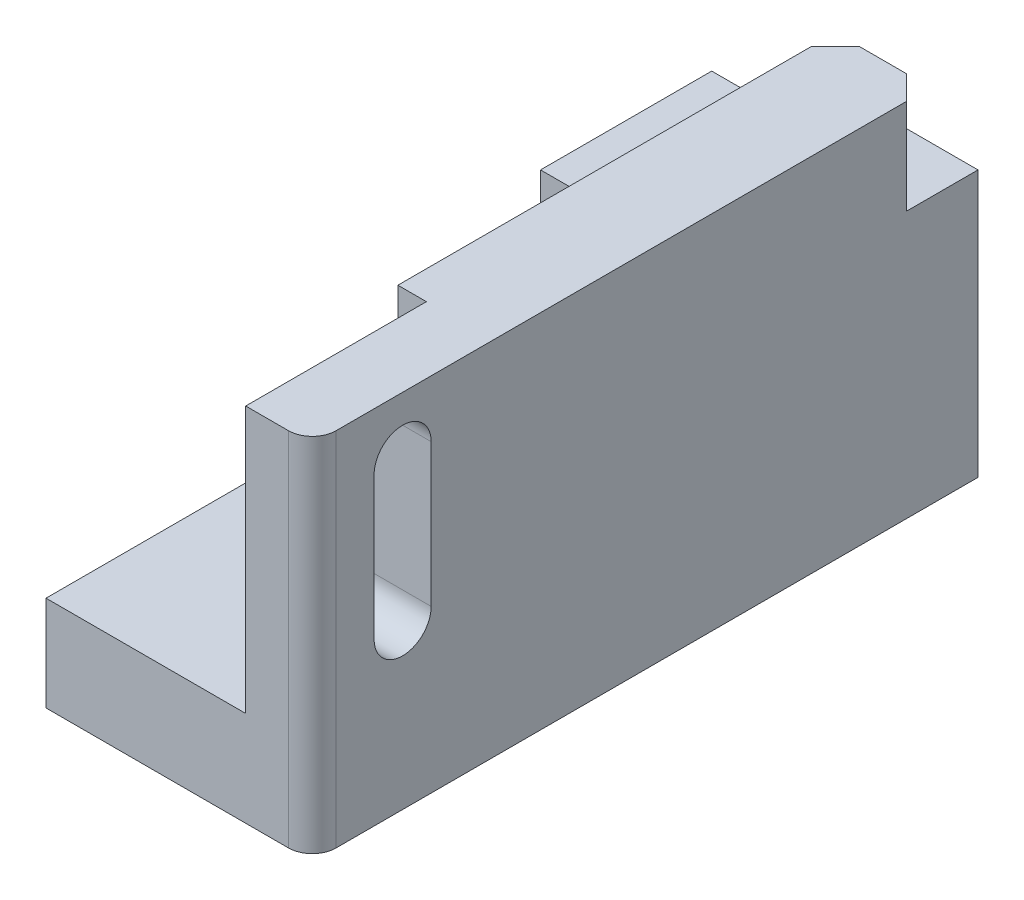
ISO-10303-21;
HEADER;
FILE_DESCRIPTION(('STEP AP214'),'2;1');
FILE_NAME('part.step','',(''),(''),'','','');
FILE_SCHEMA(('AUTOMOTIVE_DESIGN { 1 0 10303 214 1 1 1 1 }'));
ENDSEC;
DATA;
#1=APPLICATION_CONTEXT('core data for automotive mechanical design processes');
#2=APPLICATION_PROTOCOL_DEFINITION('international standard','automotive_design',2000,#1);
#3=PRODUCT_CONTEXT('',#1,'mechanical');
#4=PRODUCT('Part','Part','',(#3));
#5=PRODUCT_RELATED_PRODUCT_CATEGORY('part','',(#4));
#6=PRODUCT_DEFINITION_FORMATION('','',#4);
#7=PRODUCT_DEFINITION_CONTEXT('part definition',#1,'design');
#8=PRODUCT_DEFINITION('design','',#6,#7);
#9=PRODUCT_DEFINITION_SHAPE('','',#8);
#10=(LENGTH_UNIT() NAMED_UNIT(*) SI_UNIT(.MILLI.,.METRE.));
#11=(NAMED_UNIT(*) PLANE_ANGLE_UNIT() SI_UNIT($,.RADIAN.));
#12=(NAMED_UNIT(*) SI_UNIT($,.STERADIAN.) SOLID_ANGLE_UNIT());
#13=UNCERTAINTY_MEASURE_WITH_UNIT(LENGTH_MEASURE(1.E-05),#10,'distance_accuracy_value','');
#14=(GEOMETRIC_REPRESENTATION_CONTEXT(3) GLOBAL_UNCERTAINTY_ASSIGNED_CONTEXT((#13)) GLOBAL_UNIT_ASSIGNED_CONTEXT((#10,
#11,#12)) REPRESENTATION_CONTEXT('',''));
#15=CARTESIAN_POINT('',(0.,0.,0.));
#16=DIRECTION('',(0.,0.,1.));
#17=DIRECTION('',(1.,0.,0.));
#18=AXIS2_PLACEMENT_3D('',#15,#16,#17);
#19=CARTESIAN_POINT('',(-28.,20.,70.));
#20=DIRECTION('',(0.,0.,-1.));
#21=DIRECTION('',(-1.,0.,0.));
#22=AXIS2_PLACEMENT_3D('',#19,#20,#21);
#23=PLANE('',#22);
#24=DIRECTION('',(1.,0.,0.));
#25=VECTOR('',#24,1.);
#26=CARTESIAN_POINT('',(-28.,0.,70.));
#27=LINE('',#26,#25);
#28=CARTESIAN_POINT('',(-28.,0.,70.));
#29=VERTEX_POINT('',#28);
#30=CARTESIAN_POINT('',(23.,0.,70.));
#31=VERTEX_POINT('',#30);
#32=EDGE_CURVE('E394',#29,#31,#27,.T.);
#33=ORIENTED_EDGE('',*,*,#32,.T.);
#34=DIRECTION('',(0.,-1.,0.));
#35=VECTOR('',#34,1.);
#36=CARTESIAN_POINT('',(23.,20.,70.));
#37=LINE('',#36,#35);
#38=CARTESIAN_POINT('',(23.,76.,70.));
#39=VERTEX_POINT('',#38);
#40=EDGE_CURVE('E51',#31,#39,#37,.F.);
#41=ORIENTED_EDGE('',*,*,#40,.T.);
#42=DIRECTION('',(1.,0.,0.));
#43=VECTOR('',#42,1.);
#44=CARTESIAN_POINT('',(28.,76.,70.));
#45=LINE('',#44,#43);
#46=CARTESIAN_POINT('',(14.,76.,70.));
#47=VERTEX_POINT('',#46);
#48=EDGE_CURVE('E373',#47,#39,#45,.T.);
#49=ORIENTED_EDGE('',*,*,#48,.F.);
#50=DIRECTION('',(0.,1.,0.));
#51=VECTOR('',#50,1.);
#52=CARTESIAN_POINT('',(14.,20.,70.));
#53=LINE('',#52,#51);
#54=CARTESIAN_POINT('',(14.,20.,70.));
#55=VERTEX_POINT('',#54);
#56=EDGE_CURVE('E363',#55,#47,#53,.T.);
#57=ORIENTED_EDGE('',*,*,#56,.F.);
#58=DIRECTION('',(1.,0.,0.));
#59=VECTOR('',#58,1.);
#60=CARTESIAN_POINT('',(-28.,20.,70.));
#61=LINE('',#60,#59);
#62=CARTESIAN_POINT('',(-28.,20.,70.));
#63=VERTEX_POINT('',#62);
#64=EDGE_CURVE('E384',#63,#55,#61,.T.);
#65=ORIENTED_EDGE('',*,*,#64,.F.);
#66=DIRECTION('',(0.,-1.,0.));
#67=VECTOR('',#66,1.);
#68=CARTESIAN_POINT('',(-28.,20.,70.));
#69=LINE('',#68,#67);
#70=EDGE_CURVE('E389',#63,#29,#69,.T.);
#71=ORIENTED_EDGE('',*,*,#70,.T.);
#72=EDGE_LOOP('',(#33,#41,#49,#57,#65,#71));
#73=FACE_BOUND('',#72,.T.);
#74=ADVANCED_FACE('F43',(#73),#23,.F.);
#75=CARTESIAN_POINT('',(0.,76.,0.));
#76=DIRECTION('',(0.,-1.,0.));
#77=DIRECTION('',(0.,0.,-1.));
#78=AXIS2_PLACEMENT_3D('',#75,#76,#77);
#79=PLANE('',#78);
#80=ORIENTED_EDGE('',*,*,#48,.T.);
#81=CARTESIAN_POINT('',(23.,76.,65.));
#82=DIRECTION('',(0.,-1.,0.));
#83=DIRECTION('',(0.,0.,-1.));
#84=AXIS2_PLACEMENT_3D('',#81,#82,#83);
#85=CIRCLE('',#84,5.);
#86=CARTESIAN_POINT('',(28.,76.,65.));
#87=VERTEX_POINT('',#86);
#88=EDGE_CURVE('E11',#39,#87,#85,.F.);
#89=ORIENTED_EDGE('',*,*,#88,.T.);
#90=DIRECTION('',(0.,0.,-1.));
#91=VECTOR('',#90,1.);
#92=CARTESIAN_POINT('',(28.,76.,-70.));
#93=LINE('',#92,#91);
#94=CARTESIAN_POINT('',(28.,76.,-55.));
#95=VERTEX_POINT('',#94);
#96=EDGE_CURVE('E367',#87,#95,#93,.T.);
#97=ORIENTED_EDGE('',*,*,#96,.T.);
#98=DIRECTION('',(0.707106781186549,0.,0.707106781186546));
#99=VECTOR('',#98,1.);
#100=CARTESIAN_POINT('',(28.,76.,-55.));
#101=LINE('',#100,#99);
#102=CARTESIAN_POINT('',(23.,76.,-60.));
#103=VERTEX_POINT('',#102);
#104=EDGE_CURVE('E422',#95,#103,#101,.F.);
#105=ORIENTED_EDGE('',*,*,#104,.T.);
#106=DIRECTION('',(-1.,0.,0.));
#107=VECTOR('',#106,1.);
#108=CARTESIAN_POINT('',(73.,76.,-60.));
#109=LINE('',#108,#107);
#110=CARTESIAN_POINT('',(13.,76.,-60.));
#111=VERTEX_POINT('',#110);
#112=EDGE_CURVE('E263',#103,#111,#109,.T.);
#113=ORIENTED_EDGE('',*,*,#112,.T.);
#114=DIRECTION('',(0.707106781186549,0.,-0.707106781186546));
#115=VECTOR('',#114,1.);
#116=CARTESIAN_POINT('',(13.,76.,-60.));
#117=LINE('',#116,#115);
#118=CARTESIAN_POINT('',(8.,76.,-55.));
#119=VERTEX_POINT('',#118);
#120=EDGE_CURVE('E413',#111,#119,#117,.F.);
#121=ORIENTED_EDGE('',*,*,#120,.T.);
#122=DIRECTION('',(0.,0.,1.));
#123=VECTOR('',#122,1.);
#124=CARTESIAN_POINT('',(8.,76.,70.));
#125=LINE('',#124,#123);
#126=CARTESIAN_POINT('',(8.,76.,32.));
#127=VERTEX_POINT('',#126);
#128=EDGE_CURVE('E371',#119,#127,#125,.T.);
#129=ORIENTED_EDGE('',*,*,#128,.T.);
#130=DIRECTION('',(-1.,0.,0.));
#131=VECTOR('',#130,1.);
#132=CARTESIAN_POINT('',(0.,76.,32.));
#133=LINE('',#132,#131);
#134=CARTESIAN_POINT('',(14.,76.,32.));
#135=VERTEX_POINT('',#134);
#136=EDGE_CURVE('E352',#135,#127,#133,.T.);
#137=ORIENTED_EDGE('',*,*,#136,.F.);
#138=DIRECTION('',(0.,0.,1.));
#139=VECTOR('',#138,1.);
#140=CARTESIAN_POINT('',(14.,76.,0.));
#141=LINE('',#140,#139);
#142=EDGE_CURVE('E347',#135,#47,#141,.T.);
#143=ORIENTED_EDGE('',*,*,#142,.T.);
#144=EDGE_LOOP('',(#80,#89,#97,#105,#113,#121,#129,#137,#143));
#145=FACE_BOUND('',#144,.T.);
#146=ADVANCED_FACE('F441',(#145),#79,.F.);
#147=CARTESIAN_POINT('',(28.,20.,0.));
#148=DIRECTION('',(-1.,0.,0.));
#149=DIRECTION('',(0.,0.,1.));
#150=AXIS2_PLACEMENT_3D('',#147,#148,#149);
#151=PLANE('',#150);
#152=DIRECTION('',(0.,1.,0.));
#153=VECTOR('',#152,1.);
#154=CARTESIAN_POINT('',(28.,20.,57.));
#155=LINE('',#154,#153);
#156=CARTESIAN_POINT('',(28.,34.,57.));
#157=VERTEX_POINT('',#156);
#158=CARTESIAN_POINT('',(28.,64.,57.));
#159=VERTEX_POINT('',#158);
#160=EDGE_CURVE('E341',#157,#159,#155,.T.);
#161=ORIENTED_EDGE('',*,*,#160,.T.);
#162=CARTESIAN_POINT('',(28.,64.,51.));
#163=DIRECTION('',(-1.,0.,0.));
#164=DIRECTION('',(0.,0.,1.));
#165=AXIS2_PLACEMENT_3D('',#162,#163,#164);
#166=CIRCLE('',#165,6.00000000000001);
#167=CARTESIAN_POINT('',(28.,64.,45.));
#168=VERTEX_POINT('',#167);
#169=EDGE_CURVE('E342',#159,#168,#166,.T.);
#170=ORIENTED_EDGE('',*,*,#169,.T.);
#171=DIRECTION('',(0.,-1.,0.));
#172=VECTOR('',#171,1.);
#173=CARTESIAN_POINT('',(28.,20.,45.));
#174=LINE('',#173,#172);
#175=CARTESIAN_POINT('',(28.,34.,45.));
#176=VERTEX_POINT('',#175);
#177=EDGE_CURVE('E326',#168,#176,#174,.T.);
#178=ORIENTED_EDGE('',*,*,#177,.T.);
#179=CARTESIAN_POINT('',(28.,34.,51.));
#180=DIRECTION('',(-1.,0.,0.));
#181=DIRECTION('',(0.,0.,1.));
#182=AXIS2_PLACEMENT_3D('',#179,#180,#181);
#183=CIRCLE('',#182,6.);
#184=EDGE_CURVE('E339',#176,#157,#183,.T.);
#185=ORIENTED_EDGE('',*,*,#184,.T.);
#186=EDGE_LOOP('',(#161,#170,#178,#185));
#187=FACE_BOUND('',#186,.T.);
#188=ORIENTED_EDGE('',*,*,#96,.F.);
#189=DIRECTION('',(0.,-1.,0.));
#190=VECTOR('',#189,1.);
#191=CARTESIAN_POINT('',(28.,20.,65.));
#192=LINE('',#191,#190);
#193=CARTESIAN_POINT('',(28.,0.,65.));
#194=VERTEX_POINT('',#193);
#195=EDGE_CURVE('E429',#87,#194,#192,.T.);
#196=ORIENTED_EDGE('',*,*,#195,.T.);
#197=DIRECTION('',(0.,0.,-1.));
#198=VECTOR('',#197,1.);
#199=CARTESIAN_POINT('',(28.,0.,0.));
#200=LINE('',#199,#198);
#201=CARTESIAN_POINT('',(28.,0.,-70.));
#202=VERTEX_POINT('',#201);
#203=EDGE_CURVE('E378',#194,#202,#200,.T.);
#204=ORIENTED_EDGE('',*,*,#203,.T.);
#205=DIRECTION('',(0.,-1.,0.));
#206=VECTOR('',#205,1.);
#207=CARTESIAN_POINT('',(28.,20.,-70.));
#208=LINE('',#207,#206);
#209=CARTESIAN_POINT('',(28.,56.,-70.));
#210=VERTEX_POINT('',#209);
#211=EDGE_CURVE('E396',#210,#202,#208,.T.);
#212=ORIENTED_EDGE('',*,*,#211,.F.);
#213=DIRECTION('',(0.,0.,1.));
#214=VECTOR('',#213,1.);
#215=CARTESIAN_POINT('',(28.,56.,0.));
#216=LINE('',#215,#214);
#217=CARTESIAN_POINT('',(28.,56.,-55.));
#218=VERTEX_POINT('',#217);
#219=EDGE_CURVE('E262',#210,#218,#216,.T.);
#220=ORIENTED_EDGE('',*,*,#219,.T.);
#221=DIRECTION('',(0.,1.,0.));
#222=VECTOR('',#221,1.);
#223=CARTESIAN_POINT('',(28.,20.,-55.));
#224=LINE('',#223,#222);
#225=EDGE_CURVE('E420',#218,#95,#224,.T.);
#226=ORIENTED_EDGE('',*,*,#225,.T.);
#227=EDGE_LOOP('',(#188,#196,#204,#212,#220,#226));
#228=FACE_BOUND('',#227,.T.);
#229=ADVANCED_FACE('F450',(#187,#228),#151,.F.);
#230=CARTESIAN_POINT('',(28.,20.,-70.));
#231=DIRECTION('',(0.,0.,1.));
#232=DIRECTION('',(1.,0.,0.));
#233=AXIS2_PLACEMENT_3D('',#230,#231,#232);
#234=PLANE('',#233);
#235=DIRECTION('',(-1.,0.,0.));
#236=VECTOR('',#235,1.);
#237=CARTESIAN_POINT('',(28.,39.,-70.));
#238=LINE('',#237,#236);
#239=CARTESIAN_POINT('',(-1.49999999999999,39.,-70.));
#240=VERTEX_POINT('',#239);
#241=CARTESIAN_POINT('',(-18.5,39.,-70.));
#242=VERTEX_POINT('',#241);
#243=EDGE_CURVE('E255',#240,#242,#238,.T.);
#244=ORIENTED_EDGE('',*,*,#243,.T.);
#245=CARTESIAN_POINT('',(-18.5,33.,-70.));
#246=DIRECTION('',(0.,0.,1.));
#247=DIRECTION('',(1.,0.,0.));
#248=AXIS2_PLACEMENT_3D('',#245,#246,#247);
#249=CIRCLE('',#248,6.);
#250=CARTESIAN_POINT('',(-18.5,27.,-70.));
#251=VERTEX_POINT('',#250);
#252=EDGE_CURVE('E253',#242,#251,#249,.T.);
#253=ORIENTED_EDGE('',*,*,#252,.T.);
#254=DIRECTION('',(1.,0.,0.));
#255=VECTOR('',#254,1.);
#256=CARTESIAN_POINT('',(28.,27.,-70.));
#257=LINE('',#256,#255);
#258=CARTESIAN_POINT('',(-1.49999999999999,27.,-70.));
#259=VERTEX_POINT('',#258);
#260=EDGE_CURVE('E250',#251,#259,#257,.T.);
#261=ORIENTED_EDGE('',*,*,#260,.T.);
#262=CARTESIAN_POINT('',(-1.49999999999999,33.,-70.));
#263=DIRECTION('',(0.,0.,1.));
#264=DIRECTION('',(1.,0.,0.));
#265=AXIS2_PLACEMENT_3D('',#262,#263,#264);
#266=CIRCLE('',#265,6.);
#267=EDGE_CURVE('E227',#259,#240,#266,.T.);
#268=ORIENTED_EDGE('',*,*,#267,.T.);
#269=EDGE_LOOP('',(#244,#253,#261,#268));
#270=FACE_BOUND('',#269,.T.);
#271=DIRECTION('',(0.,-1.,0.));
#272=VECTOR('',#271,1.);
#273=CARTESIAN_POINT('',(8.,76.,-70.));
#274=LINE('',#273,#272);
#275=CARTESIAN_POINT('',(8.,56.,-70.));
#276=VERTEX_POINT('',#275);
#277=CARTESIAN_POINT('',(8.,46.,-70.));
#278=VERTEX_POINT('',#277);
#279=EDGE_CURVE('E376',#276,#278,#274,.T.);
#280=ORIENTED_EDGE('',*,*,#279,.F.);
#281=DIRECTION('',(-1.,0.,0.));
#282=VECTOR('',#281,1.);
#283=CARTESIAN_POINT('',(73.,56.,-70.));
#284=LINE('',#283,#282);
#285=EDGE_CURVE('E257',#210,#276,#284,.T.);
#286=ORIENTED_EDGE('',*,*,#285,.F.);
#287=ORIENTED_EDGE('',*,*,#211,.T.);
#288=DIRECTION('',(-1.,0.,0.));
#289=VECTOR('',#288,1.);
#290=CARTESIAN_POINT('',(28.,0.,-70.));
#291=LINE('',#290,#289);
#292=CARTESIAN_POINT('',(-28.,0.,-70.));
#293=VERTEX_POINT('',#292);
#294=EDGE_CURVE('E390',#202,#293,#291,.T.);
#295=ORIENTED_EDGE('',*,*,#294,.T.);
#296=DIRECTION('',(0.,-1.,0.));
#297=VECTOR('',#296,1.);
#298=CARTESIAN_POINT('',(-28.,20.,-70.));
#299=LINE('',#298,#297);
#300=CARTESIAN_POINT('',(-28.,46.,-70.));
#301=VERTEX_POINT('',#300);
#302=EDGE_CURVE('E399',#301,#293,#299,.T.);
#303=ORIENTED_EDGE('',*,*,#302,.F.);
#304=DIRECTION('',(-1.,0.,0.));
#305=VECTOR('',#304,1.);
#306=CARTESIAN_POINT('',(8.,46.,-70.));
#307=LINE('',#306,#305);
#308=EDGE_CURVE('E307',#278,#301,#307,.T.);
#309=ORIENTED_EDGE('',*,*,#308,.F.);
#310=EDGE_LOOP('',(#280,#286,#287,#295,#303,#309));
#311=FACE_BOUND('',#310,.T.);
#312=ADVANCED_FACE('F452',(#270,#311),#234,.F.);
#313=CARTESIAN_POINT('',(-28.,20.,-70.));
#314=DIRECTION('',(1.,0.,0.));
#315=DIRECTION('',(0.,0.,-1.));
#316=AXIS2_PLACEMENT_3D('',#313,#314,#315);
#317=PLANE('',#316);
#318=DIRECTION('',(0.,0.,1.));
#319=VECTOR('',#318,1.);
#320=CARTESIAN_POINT('',(-28.,20.,-70.));
#321=LINE('',#320,#319);
#322=CARTESIAN_POINT('',(-28.,20.,11.));
#323=VERTEX_POINT('',#322);
#324=EDGE_CURVE('E381',#323,#63,#321,.T.);
#325=ORIENTED_EDGE('',*,*,#324,.F.);
#326=DIRECTION('',(0.,1.,0.));
#327=VECTOR('',#326,1.);
#328=CARTESIAN_POINT('',(-28.,10.,11.));
#329=LINE('',#328,#327);
#330=CARTESIAN_POINT('',(-28.,10.,11.));
#331=VERTEX_POINT('',#330);
#332=EDGE_CURVE('E276',#331,#323,#329,.T.);
#333=ORIENTED_EDGE('',*,*,#332,.F.);
#334=DIRECTION('',(0.,0.,1.));
#335=VECTOR('',#334,1.);
#336=CARTESIAN_POINT('',(-28.,10.,-19.));
#337=LINE('',#336,#335);
#338=CARTESIAN_POINT('',(-28.,10.,-19.));
#339=VERTEX_POINT('',#338);
#340=EDGE_CURVE('E287',#339,#331,#337,.T.);
#341=ORIENTED_EDGE('',*,*,#340,.F.);
#342=DIRECTION('',(0.,-1.,0.));
#343=VECTOR('',#342,1.);
#344=CARTESIAN_POINT('',(-28.,20.,-19.));
#345=LINE('',#344,#343);
#346=CARTESIAN_POINT('',(-28.,20.,-19.));
#347=VERTEX_POINT('',#346);
#348=EDGE_CURVE('E275',#347,#339,#345,.T.);
#349=ORIENTED_EDGE('',*,*,#348,.F.);
#350=CARTESIAN_POINT('',(-28.,20.,-34.));
#351=VERTEX_POINT('',#350);
#352=EDGE_CURVE('E379',#351,#347,#321,.T.);
#353=ORIENTED_EDGE('',*,*,#352,.F.);
#354=DIRECTION('',(0.,1.,0.));
#355=VECTOR('',#354,1.);
#356=CARTESIAN_POINT('',(-28.,46.,-34.));
#357=LINE('',#356,#355);
#358=CARTESIAN_POINT('',(-28.,46.,-34.));
#359=VERTEX_POINT('',#358);
#360=EDGE_CURVE('E294',#351,#359,#357,.T.);
#361=ORIENTED_EDGE('',*,*,#360,.T.);
#362=DIRECTION('',(0.,0.,-1.));
#363=VECTOR('',#362,1.);
#364=CARTESIAN_POINT('',(-28.,46.,-70.));
#365=LINE('',#364,#363);
#366=EDGE_CURVE('E304',#359,#301,#365,.T.);
#367=ORIENTED_EDGE('',*,*,#366,.T.);
#368=ORIENTED_EDGE('',*,*,#302,.T.);
#369=DIRECTION('',(0.,0.,1.));
#370=VECTOR('',#369,1.);
#371=CARTESIAN_POINT('',(-28.,0.,-70.));
#372=LINE('',#371,#370);
#373=EDGE_CURVE('E387',#293,#29,#372,.T.);
#374=ORIENTED_EDGE('',*,*,#373,.T.);
#375=ORIENTED_EDGE('',*,*,#70,.F.);
#376=EDGE_LOOP('',(#325,#333,#341,#349,#353,#361,#367,#368,#374,#375));
#377=FACE_BOUND('',#376,.T.);
#378=ADVANCED_FACE('F456',(#377),#317,.F.);
#379=CARTESIAN_POINT('',(0.,20.,0.));
#380=DIRECTION('',(0.,1.,0.));
#381=DIRECTION('',(0.,0.,1.));
#382=AXIS2_PLACEMENT_3D('',#379,#380,#381);
#383=PLANE('',#382);
#384=DIRECTION('',(-1.,0.,0.));
#385=VECTOR('',#384,1.);
#386=CARTESIAN_POINT('',(-5.99999999999999,20.,11.));
#387=LINE('',#386,#385);
#388=CARTESIAN_POINT('',(-5.99999999999999,20.,11.));
#389=VERTEX_POINT('',#388);
#390=EDGE_CURVE('E292',#389,#323,#387,.T.);
#391=ORIENTED_EDGE('',*,*,#390,.T.);
#392=ORIENTED_EDGE('',*,*,#324,.T.);
#393=ORIENTED_EDGE('',*,*,#64,.T.);
#394=DIRECTION('',(0.,0.,1.));
#395=VECTOR('',#394,1.);
#396=CARTESIAN_POINT('',(14.,20.,0.));
#397=LINE('',#396,#395);
#398=CARTESIAN_POINT('',(14.,20.,32.));
#399=VERTEX_POINT('',#398);
#400=EDGE_CURVE('E350',#399,#55,#397,.T.);
#401=ORIENTED_EDGE('',*,*,#400,.F.);
#402=DIRECTION('',(-1.,0.,0.));
#403=VECTOR('',#402,1.);
#404=CARTESIAN_POINT('',(0.,20.,32.));
#405=LINE('',#404,#403);
#406=CARTESIAN_POINT('',(8.,20.,32.));
#407=VERTEX_POINT('',#406);
#408=EDGE_CURVE('E354',#399,#407,#405,.T.);
#409=ORIENTED_EDGE('',*,*,#408,.T.);
#410=DIRECTION('',(0.,0.,1.));
#411=VECTOR('',#410,1.);
#412=CARTESIAN_POINT('',(8.,20.,70.));
#413=LINE('',#412,#411);
#414=CARTESIAN_POINT('',(8.,20.,-34.));
#415=VERTEX_POINT('',#414);
#416=EDGE_CURVE('E361',#415,#407,#413,.T.);
#417=ORIENTED_EDGE('',*,*,#416,.F.);
#418=DIRECTION('',(1.,0.,0.));
#419=VECTOR('',#418,1.);
#420=CARTESIAN_POINT('',(0.,20.,-34.));
#421=LINE('',#420,#419);
#422=EDGE_CURVE('E315',#351,#415,#421,.T.);
#423=ORIENTED_EDGE('',*,*,#422,.F.);
#424=ORIENTED_EDGE('',*,*,#352,.T.);
#425=DIRECTION('',(-1.,0.,0.));
#426=VECTOR('',#425,1.);
#427=CARTESIAN_POINT('',(-5.99999999999999,20.,-19.));
#428=LINE('',#427,#426);
#429=CARTESIAN_POINT('',(-5.99999999999999,20.,-19.));
#430=VERTEX_POINT('',#429);
#431=EDGE_CURVE('E281',#430,#347,#428,.T.);
#432=ORIENTED_EDGE('',*,*,#431,.F.);
#433=DIRECTION('',(0.,0.,-1.));
#434=VECTOR('',#433,1.);
#435=CARTESIAN_POINT('',(-5.99999999999999,20.,11.));
#436=LINE('',#435,#434);
#437=EDGE_CURVE('E271',#389,#430,#436,.T.);
#438=ORIENTED_EDGE('',*,*,#437,.F.);
#439=EDGE_LOOP('',(#391,#392,#393,#401,#409,#417,#423,#424,#432,#438));
#440=FACE_BOUND('',#439,.T.);
#441=ADVANCED_FACE('F500',(#440),#383,.T.);
#442=CARTESIAN_POINT('',(0.,0.,0.));
#443=DIRECTION('',(0.,1.,0.));
#444=DIRECTION('',(0.,0.,1.));
#445=AXIS2_PLACEMENT_3D('',#442,#443,#444);
#446=PLANE('',#445);
#447=CARTESIAN_POINT('',(-17.,0.,-4.00000000000001));
#448=DIRECTION('',(0.,1.,0.));
#449=DIRECTION('',(0.,0.,1.));
#450=AXIS2_PLACEMENT_3D('',#447,#448,#449);
#451=CIRCLE('',#450,6.);
#452=CARTESIAN_POINT('',(-17.,0.,1.99999999999999));
#453=VERTEX_POINT('',#452);
#454=EDGE_CURVE('E270',#453,#453,#451,.T.);
#455=ORIENTED_EDGE('',*,*,#454,.T.);
#456=EDGE_LOOP('',(#455));
#457=FACE_BOUND('',#456,.T.);
#458=ORIENTED_EDGE('',*,*,#203,.F.);
#459=CARTESIAN_POINT('',(23.,0.,65.));
#460=DIRECTION('',(0.,1.,0.));
#461=DIRECTION('',(0.,0.,1.));
#462=AXIS2_PLACEMENT_3D('',#459,#460,#461);
#463=CIRCLE('',#462,5.);
#464=EDGE_CURVE('E435',#194,#31,#463,.F.);
#465=ORIENTED_EDGE('',*,*,#464,.T.);
#466=ORIENTED_EDGE('',*,*,#32,.F.);
#467=ORIENTED_EDGE('',*,*,#373,.F.);
#468=ORIENTED_EDGE('',*,*,#294,.F.);
#469=EDGE_LOOP('',(#458,#465,#466,#467,#468));
#470=FACE_BOUND('',#469,.T.);
#471=ADVANCED_FACE('F454',(#457,#470),#446,.F.);
#472=CARTESIAN_POINT('',(8.,76.,70.));
#473=DIRECTION('',(1.,0.,0.));
#474=DIRECTION('',(0.,0.,-1.));
#475=AXIS2_PLACEMENT_3D('',#472,#473,#474);
#476=PLANE('',#475);
#477=ORIENTED_EDGE('',*,*,#128,.F.);
#478=DIRECTION('',(0.,-1.,0.));
#479=VECTOR('',#478,1.);
#480=CARTESIAN_POINT('',(8.,76.,-55.));
#481=LINE('',#480,#479);
#482=CARTESIAN_POINT('',(8.,56.,-55.));
#483=VERTEX_POINT('',#482);
#484=EDGE_CURVE('E412',#119,#483,#481,.T.);
#485=ORIENTED_EDGE('',*,*,#484,.T.);
#486=DIRECTION('',(0.,0.,1.));
#487=VECTOR('',#486,1.);
#488=CARTESIAN_POINT('',(8.,56.,-70.));
#489=LINE('',#488,#487);
#490=EDGE_CURVE('E260',#276,#483,#489,.T.);
#491=ORIENTED_EDGE('',*,*,#490,.F.);
#492=ORIENTED_EDGE('',*,*,#279,.T.);
#493=DIRECTION('',(0.,0.,-1.));
#494=VECTOR('',#493,1.);
#495=CARTESIAN_POINT('',(8.,46.,-70.));
#496=LINE('',#495,#494);
#497=CARTESIAN_POINT('',(8.,46.,-34.));
#498=VERTEX_POINT('',#497);
#499=EDGE_CURVE('E301',#498,#278,#496,.T.);
#500=ORIENTED_EDGE('',*,*,#499,.F.);
#501=DIRECTION('',(0.,-1.,0.));
#502=VECTOR('',#501,1.);
#503=CARTESIAN_POINT('',(8.,76.,-34.));
#504=LINE('',#503,#502);
#505=EDGE_CURVE('E401',#498,#415,#504,.T.);
#506=ORIENTED_EDGE('',*,*,#505,.T.);
#507=ORIENTED_EDGE('',*,*,#416,.T.);
#508=DIRECTION('',(0.,1.,0.));
#509=VECTOR('',#508,1.);
#510=CARTESIAN_POINT('',(8.,20.,32.));
#511=LINE('',#510,#509);
#512=EDGE_CURVE('E364',#407,#127,#511,.T.);
#513=ORIENTED_EDGE('',*,*,#512,.T.);
#514=EDGE_LOOP('',(#477,#485,#491,#492,#500,#506,#507,#513));
#515=FACE_BOUND('',#514,.T.);
#516=ADVANCED_FACE('F474',(#515),#476,.F.);
#517=CARTESIAN_POINT('',(14.,20.,0.));
#518=DIRECTION('',(-1.,0.,0.));
#519=DIRECTION('',(0.,0.,1.));
#520=AXIS2_PLACEMENT_3D('',#517,#518,#519);
#521=PLANE('',#520);
#522=CARTESIAN_POINT('',(14.,64.,51.));
#523=DIRECTION('',(-1.,0.,0.));
#524=DIRECTION('',(0.,0.,1.));
#525=AXIS2_PLACEMENT_3D('',#522,#523,#524);
#526=CIRCLE('',#525,6.00000000000001);
#527=CARTESIAN_POINT('',(14.,64.,57.));
#528=VERTEX_POINT('',#527);
#529=CARTESIAN_POINT('',(14.,64.,45.));
#530=VERTEX_POINT('',#529);
#531=EDGE_CURVE('E317',#528,#530,#526,.T.);
#532=ORIENTED_EDGE('',*,*,#531,.F.);
#533=DIRECTION('',(0.,1.,0.));
#534=VECTOR('',#533,1.);
#535=CARTESIAN_POINT('',(14.,64.,57.));
#536=LINE('',#535,#534);
#537=CARTESIAN_POINT('',(14.,34.,57.));
#538=VERTEX_POINT('',#537);
#539=EDGE_CURVE('E323',#538,#528,#536,.T.);
#540=ORIENTED_EDGE('',*,*,#539,.F.);
#541=CARTESIAN_POINT('',(14.,34.,51.));
#542=DIRECTION('',(-1.,0.,0.));
#543=DIRECTION('',(0.,0.,1.));
#544=AXIS2_PLACEMENT_3D('',#541,#542,#543);
#545=CIRCLE('',#544,6.);
#546=CARTESIAN_POINT('',(14.,34.,45.));
#547=VERTEX_POINT('',#546);
#548=EDGE_CURVE('E324',#547,#538,#545,.T.);
#549=ORIENTED_EDGE('',*,*,#548,.F.);
#550=DIRECTION('',(0.,-1.,0.));
#551=VECTOR('',#550,1.);
#552=CARTESIAN_POINT('',(14.,34.,45.));
#553=LINE('',#552,#551);
#554=EDGE_CURVE('E319',#530,#547,#553,.T.);
#555=ORIENTED_EDGE('',*,*,#554,.F.);
#556=EDGE_LOOP('',(#532,#540,#549,#555));
#557=FACE_BOUND('',#556,.T.);
#558=ORIENTED_EDGE('',*,*,#142,.F.);
#559=DIRECTION('',(0.,1.,0.));
#560=VECTOR('',#559,1.);
#561=CARTESIAN_POINT('',(14.,20.,32.));
#562=LINE('',#561,#560);
#563=EDGE_CURVE('E358',#399,#135,#562,.T.);
#564=ORIENTED_EDGE('',*,*,#563,.F.);
#565=ORIENTED_EDGE('',*,*,#400,.T.);
#566=ORIENTED_EDGE('',*,*,#56,.T.);
#567=EDGE_LOOP('',(#558,#564,#565,#566));
#568=FACE_BOUND('',#567,.T.);
#569=ADVANCED_FACE('F501',(#557,#568),#521,.T.);
#570=CARTESIAN_POINT('',(0.,20.,32.));
#571=DIRECTION('',(0.,0.,-1.));
#572=DIRECTION('',(-1.,0.,0.));
#573=AXIS2_PLACEMENT_3D('',#570,#571,#572);
#574=PLANE('',#573);
#575=ORIENTED_EDGE('',*,*,#136,.T.);
#576=ORIENTED_EDGE('',*,*,#512,.F.);
#577=ORIENTED_EDGE('',*,*,#408,.F.);
#578=ORIENTED_EDGE('',*,*,#563,.T.);
#579=EDGE_LOOP('',(#575,#576,#577,#578));
#580=FACE_BOUND('',#579,.T.);
#581=ADVANCED_FACE('F494',(#580),#574,.F.);
#582=CARTESIAN_POINT('',(70.,64.,51.));
#583=DIRECTION('',(-1.,0.,0.));
#584=DIRECTION('',(0.,0.,1.));
#585=AXIS2_PLACEMENT_3D('',#582,#583,#584);
#586=CYLINDRICAL_SURFACE('',#585,6.00000000000001);
#587=DIRECTION('',(-1.,0.,0.));
#588=VECTOR('',#587,1.);
#589=CARTESIAN_POINT('',(70.,64.,57.));
#590=LINE('',#589,#588);
#591=EDGE_CURVE('E327',#159,#528,#590,.T.);
#592=ORIENTED_EDGE('',*,*,#591,.T.);
#593=ORIENTED_EDGE('',*,*,#531,.T.);
#594=DIRECTION('',(-1.,0.,0.));
#595=VECTOR('',#594,1.);
#596=CARTESIAN_POINT('',(70.,64.,45.));
#597=LINE('',#596,#595);
#598=EDGE_CURVE('E329',#168,#530,#597,.T.);
#599=ORIENTED_EDGE('',*,*,#598,.F.);
#600=ORIENTED_EDGE('',*,*,#169,.F.);
#601=EDGE_LOOP('',(#592,#593,#599,#600));
#602=FACE_BOUND('',#601,.T.);
#603=ADVANCED_FACE('F706',(#602),#586,.F.);
#604=CARTESIAN_POINT('',(70.,64.,57.));
#605=DIRECTION('',(0.,0.,1.));
#606=DIRECTION('',(0.,-1.,0.));
#607=AXIS2_PLACEMENT_3D('',#604,#605,#606);
#608=PLANE('',#607);
#609=DIRECTION('',(-1.,0.,0.));
#610=VECTOR('',#609,1.);
#611=CARTESIAN_POINT('',(70.,34.,57.));
#612=LINE('',#611,#610);
#613=EDGE_CURVE('E333',#157,#538,#612,.T.);
#614=ORIENTED_EDGE('',*,*,#613,.T.);
#615=ORIENTED_EDGE('',*,*,#539,.T.);
#616=ORIENTED_EDGE('',*,*,#591,.F.);
#617=ORIENTED_EDGE('',*,*,#160,.F.);
#618=EDGE_LOOP('',(#614,#615,#616,#617));
#619=FACE_BOUND('',#618,.T.);
#620=ADVANCED_FACE('F699',(#619),#608,.F.);
#621=CARTESIAN_POINT('',(70.,34.,51.));
#622=DIRECTION('',(-1.,0.,0.));
#623=DIRECTION('',(0.,0.,1.));
#624=AXIS2_PLACEMENT_3D('',#621,#622,#623);
#625=CYLINDRICAL_SURFACE('',#624,6.);
#626=DIRECTION('',(-1.,0.,0.));
#627=VECTOR('',#626,1.);
#628=CARTESIAN_POINT('',(70.,34.,45.));
#629=LINE('',#628,#627);
#630=EDGE_CURVE('E332',#176,#547,#629,.T.);
#631=ORIENTED_EDGE('',*,*,#630,.T.);
#632=ORIENTED_EDGE('',*,*,#548,.T.);
#633=ORIENTED_EDGE('',*,*,#613,.F.);
#634=ORIENTED_EDGE('',*,*,#184,.F.);
#635=EDGE_LOOP('',(#631,#632,#633,#634));
#636=FACE_BOUND('',#635,.T.);
#637=ADVANCED_FACE('F687',(#636),#625,.F.);
#638=CARTESIAN_POINT('',(70.,34.,45.));
#639=DIRECTION('',(0.,0.,-1.));
#640=DIRECTION('',(0.,1.,0.));
#641=AXIS2_PLACEMENT_3D('',#638,#639,#640);
#642=PLANE('',#641);
#643=ORIENTED_EDGE('',*,*,#598,.T.);
#644=ORIENTED_EDGE('',*,*,#554,.T.);
#645=ORIENTED_EDGE('',*,*,#630,.F.);
#646=ORIENTED_EDGE('',*,*,#177,.F.);
#647=EDGE_LOOP('',(#643,#644,#645,#646));
#648=FACE_BOUND('',#647,.T.);
#649=ADVANCED_FACE('F525',(#648),#642,.F.);
#650=CARTESIAN_POINT('',(8.,46.,-70.));
#651=DIRECTION('',(0.,1.,0.));
#652=DIRECTION('',(0.,0.,1.));
#653=AXIS2_PLACEMENT_3D('',#650,#651,#652);
#654=PLANE('',#653);
#655=ORIENTED_EDGE('',*,*,#366,.F.);
#656=DIRECTION('',(-1.,0.,0.));
#657=VECTOR('',#656,1.);
#658=CARTESIAN_POINT('',(8.,46.,-34.));
#659=LINE('',#658,#657);
#660=EDGE_CURVE('E302',#498,#359,#659,.T.);
#661=ORIENTED_EDGE('',*,*,#660,.F.);
#662=ORIENTED_EDGE('',*,*,#499,.T.);
#663=ORIENTED_EDGE('',*,*,#308,.T.);
#664=EDGE_LOOP('',(#655,#661,#662,#663));
#665=FACE_BOUND('',#664,.T.);
#666=ADVANCED_FACE('F467',(#665),#654,.T.);
#667=CARTESIAN_POINT('',(8.,46.,-34.));
#668=DIRECTION('',(0.,0.,1.));
#669=DIRECTION('',(1.,0.,0.));
#670=AXIS2_PLACEMENT_3D('',#667,#668,#669);
#671=PLANE('',#670);
#672=CARTESIAN_POINT('',(-18.5,33.,-34.));
#673=DIRECTION('',(0.,0.,1.));
#674=DIRECTION('',(1.,0.,0.));
#675=AXIS2_PLACEMENT_3D('',#672,#673,#674);
#676=CIRCLE('',#675,6.);
#677=CARTESIAN_POINT('',(-18.5,39.,-34.));
#678=VERTEX_POINT('',#677);
#679=CARTESIAN_POINT('',(-18.5,27.,-34.));
#680=VERTEX_POINT('',#679);
#681=EDGE_CURVE('E68',#678,#680,#676,.T.);
#682=ORIENTED_EDGE('',*,*,#681,.F.);
#683=DIRECTION('',(-1.,0.,0.));
#684=VECTOR('',#683,1.);
#685=CARTESIAN_POINT('',(-18.5,39.,-34.));
#686=LINE('',#685,#684);
#687=CARTESIAN_POINT('',(-1.49999999999999,39.,-34.));
#688=VERTEX_POINT('',#687);
#689=EDGE_CURVE('E239',#688,#678,#686,.T.);
#690=ORIENTED_EDGE('',*,*,#689,.F.);
#691=CARTESIAN_POINT('',(-1.49999999999999,33.,-34.));
#692=DIRECTION('',(0.,0.,1.));
#693=DIRECTION('',(1.,0.,0.));
#694=AXIS2_PLACEMENT_3D('',#691,#692,#693);
#695=CIRCLE('',#694,6.);
#696=CARTESIAN_POINT('',(-1.49999999999999,27.,-34.));
#697=VERTEX_POINT('',#696);
#698=EDGE_CURVE('E225',#697,#688,#695,.T.);
#699=ORIENTED_EDGE('',*,*,#698,.F.);
#700=DIRECTION('',(1.,0.,0.));
#701=VECTOR('',#700,1.);
#702=CARTESIAN_POINT('',(-18.5,27.,-34.));
#703=LINE('',#702,#701);
#704=EDGE_CURVE('E231',#680,#697,#703,.T.);
#705=ORIENTED_EDGE('',*,*,#704,.F.);
#706=EDGE_LOOP('',(#682,#690,#699,#705));
#707=FACE_BOUND('',#706,.T.);
#708=ORIENTED_EDGE('',*,*,#360,.F.);
#709=ORIENTED_EDGE('',*,*,#422,.T.);
#710=ORIENTED_EDGE('',*,*,#505,.F.);
#711=ORIENTED_EDGE('',*,*,#660,.T.);
#712=EDGE_LOOP('',(#708,#709,#710,#711));
#713=FACE_BOUND('',#712,.T.);
#714=ADVANCED_FACE('F240',(#707,#713),#671,.T.);
#715=CARTESIAN_POINT('',(-5.99999999999999,10.,11.));
#716=DIRECTION('',(0.,0.,1.));
#717=DIRECTION('',(1.,0.,0.));
#718=AXIS2_PLACEMENT_3D('',#715,#716,#717);
#719=PLANE('',#718);
#720=ORIENTED_EDGE('',*,*,#332,.T.);
#721=ORIENTED_EDGE('',*,*,#390,.F.);
#722=DIRECTION('',(0.,1.,0.));
#723=VECTOR('',#722,1.);
#724=CARTESIAN_POINT('',(-5.99999999999999,10.,11.));
#725=LINE('',#724,#723);
#726=CARTESIAN_POINT('',(-5.99999999999999,10.,11.));
#727=VERTEX_POINT('',#726);
#728=EDGE_CURVE('E282',#727,#389,#725,.T.);
#729=ORIENTED_EDGE('',*,*,#728,.F.);
#730=DIRECTION('',(-1.,0.,0.));
#731=VECTOR('',#730,1.);
#732=CARTESIAN_POINT('',(-5.99999999999999,10.,11.));
#733=LINE('',#732,#731);
#734=EDGE_CURVE('E298',#727,#331,#733,.T.);
#735=ORIENTED_EDGE('',*,*,#734,.T.);
#736=EDGE_LOOP('',(#720,#721,#729,#735));
#737=FACE_BOUND('',#736,.T.);
#738=ADVANCED_FACE('F508',(#737),#719,.F.);
#739=CARTESIAN_POINT('',(-5.99999999999999,10.,-19.));
#740=DIRECTION('',(0.,-1.,0.));
#741=DIRECTION('',(0.,0.,-1.));
#742=AXIS2_PLACEMENT_3D('',#739,#740,#741);
#743=PLANE('',#742);
#744=CARTESIAN_POINT('',(-17.,10.,-4.00000000000001));
#745=DIRECTION('',(0.,-1.,0.));
#746=DIRECTION('',(0.,0.,-1.));
#747=AXIS2_PLACEMENT_3D('',#744,#745,#746);
#748=CIRCLE('',#747,6.);
#749=CARTESIAN_POINT('',(-17.,10.,-10.));
#750=VERTEX_POINT('',#749);
#751=EDGE_CURVE('E267',#750,#750,#748,.T.);
#752=ORIENTED_EDGE('',*,*,#751,.T.);
#753=EDGE_LOOP('',(#752));
#754=FACE_BOUND('',#753,.T.);
#755=ORIENTED_EDGE('',*,*,#340,.T.);
#756=ORIENTED_EDGE('',*,*,#734,.F.);
#757=DIRECTION('',(0.,0.,1.));
#758=VECTOR('',#757,1.);
#759=CARTESIAN_POINT('',(-5.99999999999999,10.,-19.));
#760=LINE('',#759,#758);
#761=CARTESIAN_POINT('',(-5.99999999999999,10.,-19.));
#762=VERTEX_POINT('',#761);
#763=EDGE_CURVE('E277',#762,#727,#760,.T.);
#764=ORIENTED_EDGE('',*,*,#763,.F.);
#765=DIRECTION('',(-1.,0.,0.));
#766=VECTOR('',#765,1.);
#767=CARTESIAN_POINT('',(-5.99999999999999,10.,-19.));
#768=LINE('',#767,#766);
#769=EDGE_CURVE('E296',#762,#339,#768,.T.);
#770=ORIENTED_EDGE('',*,*,#769,.T.);
#771=EDGE_LOOP('',(#755,#756,#764,#770));
#772=FACE_BOUND('',#771,.T.);
#773=ADVANCED_FACE('F515',(#754,#772),#743,.F.);
#774=CARTESIAN_POINT('',(-5.99999999999999,20.,-19.));
#775=DIRECTION('',(0.,0.,-1.));
#776=DIRECTION('',(-1.,0.,0.));
#777=AXIS2_PLACEMENT_3D('',#774,#775,#776);
#778=PLANE('',#777);
#779=ORIENTED_EDGE('',*,*,#348,.T.);
#780=ORIENTED_EDGE('',*,*,#769,.F.);
#781=DIRECTION('',(0.,-1.,0.));
#782=VECTOR('',#781,1.);
#783=CARTESIAN_POINT('',(-5.99999999999999,20.,-19.));
#784=LINE('',#783,#782);
#785=EDGE_CURVE('E279',#430,#762,#784,.T.);
#786=ORIENTED_EDGE('',*,*,#785,.F.);
#787=ORIENTED_EDGE('',*,*,#431,.T.);
#788=EDGE_LOOP('',(#779,#780,#786,#787));
#789=FACE_BOUND('',#788,.T.);
#790=ADVANCED_FACE('F579',(#789),#778,.F.);
#791=CARTESIAN_POINT('',(-5.99999999999999,0.,0.));
#792=DIRECTION('',(-1.,0.,0.));
#793=DIRECTION('',(0.,0.,1.));
#794=AXIS2_PLACEMENT_3D('',#791,#792,#793);
#795=PLANE('',#794);
#796=ORIENTED_EDGE('',*,*,#437,.T.);
#797=ORIENTED_EDGE('',*,*,#785,.T.);
#798=ORIENTED_EDGE('',*,*,#763,.T.);
#799=ORIENTED_EDGE('',*,*,#728,.T.);
#800=EDGE_LOOP('',(#796,#797,#798,#799));
#801=FACE_BOUND('',#800,.T.);
#802=ADVANCED_FACE('F574',(#801),#795,.T.);
#803=CARTESIAN_POINT('',(-17.,-45.,-4.00000000000001));
#804=DIRECTION('',(0.,1.,0.));
#805=DIRECTION('',(0.,0.,1.));
#806=AXIS2_PLACEMENT_3D('',#803,#804,#805);
#807=CYLINDRICAL_SURFACE('',#806,6.);
#808=ORIENTED_EDGE('',*,*,#751,.F.);
#809=EDGE_LOOP('',(#808));
#810=FACE_BOUND('',#809,.T.);
#811=ORIENTED_EDGE('',*,*,#454,.F.);
#812=EDGE_LOOP('',(#811));
#813=FACE_BOUND('',#812,.T.);
#814=ADVANCED_FACE('F571',(#810,#813),#807,.F.);
#815=CARTESIAN_POINT('',(73.,56.,-60.));
#816=DIRECTION('',(0.,0.,1.));
#817=DIRECTION('',(1.,0.,0.));
#818=AXIS2_PLACEMENT_3D('',#815,#816,#817);
#819=PLANE('',#818);
#820=ORIENTED_EDGE('',*,*,#112,.F.);
#821=DIRECTION('',(0.,-1.,0.));
#822=VECTOR('',#821,1.);
#823=CARTESIAN_POINT('',(23.,56.,-60.));
#824=LINE('',#823,#822);
#825=CARTESIAN_POINT('',(23.,56.,-60.));
#826=VERTEX_POINT('',#825);
#827=EDGE_CURVE('E425',#103,#826,#824,.T.);
#828=ORIENTED_EDGE('',*,*,#827,.T.);
#829=DIRECTION('',(-1.,0.,0.));
#830=VECTOR('',#829,1.);
#831=CARTESIAN_POINT('',(73.,56.,-60.));
#832=LINE('',#831,#830);
#833=CARTESIAN_POINT('',(13.,56.,-60.));
#834=VERTEX_POINT('',#833);
#835=EDGE_CURVE('E265',#826,#834,#832,.T.);
#836=ORIENTED_EDGE('',*,*,#835,.T.);
#837=DIRECTION('',(0.,1.,0.));
#838=VECTOR('',#837,1.);
#839=CARTESIAN_POINT('',(13.,56.,-60.));
#840=LINE('',#839,#838);
#841=EDGE_CURVE('E409',#834,#111,#840,.T.);
#842=ORIENTED_EDGE('',*,*,#841,.T.);
#843=EDGE_LOOP('',(#820,#828,#836,#842));
#844=FACE_BOUND('',#843,.T.);
#845=ADVANCED_FACE('F487',(#844),#819,.F.);
#846=CARTESIAN_POINT('',(73.,56.,-70.));
#847=DIRECTION('',(0.,-1.,0.));
#848=DIRECTION('',(0.,0.,-1.));
#849=AXIS2_PLACEMENT_3D('',#846,#847,#848);
#850=PLANE('',#849);
#851=ORIENTED_EDGE('',*,*,#285,.T.);
#852=ORIENTED_EDGE('',*,*,#490,.T.);
#853=DIRECTION('',(-0.707106781186549,0.,0.707106781186546));
#854=VECTOR('',#853,1.);
#855=CARTESIAN_POINT('',(48.0000000000001,56.,-95.));
#856=LINE('',#855,#854);
#857=EDGE_CURVE('E418',#483,#834,#856,.F.);
#858=ORIENTED_EDGE('',*,*,#857,.T.);
#859=ORIENTED_EDGE('',*,*,#835,.F.);
#860=DIRECTION('',(-0.707106781186549,0.,-0.707106781186546));
#861=VECTOR('',#860,1.);
#862=CARTESIAN_POINT('',(43.0000000000001,56.,-40.));
#863=LINE('',#862,#861);
#864=EDGE_CURVE('E428',#826,#218,#863,.F.);
#865=ORIENTED_EDGE('',*,*,#864,.T.);
#866=ORIENTED_EDGE('',*,*,#219,.F.);
#867=EDGE_LOOP('',(#851,#852,#858,#859,#865,#866));
#868=FACE_BOUND('',#867,.T.);
#869=ADVANCED_FACE('F472',(#868),#850,.F.);
#870=CARTESIAN_POINT('',(13.,56.,-60.));
#871=DIRECTION('',(0.707106781186546,0.,0.707106781186549));
#872=DIRECTION('',(0.,1.,0.));
#873=AXIS2_PLACEMENT_3D('',#870,#871,#872);
#874=PLANE('',#873);
#875=ORIENTED_EDGE('',*,*,#857,.F.);
#876=ORIENTED_EDGE('',*,*,#484,.F.);
#877=ORIENTED_EDGE('',*,*,#120,.F.);
#878=ORIENTED_EDGE('',*,*,#841,.F.);
#879=EDGE_LOOP('',(#875,#876,#877,#878));
#880=FACE_BOUND('',#879,.T.);
#881=ADVANCED_FACE('F490',(#880),#874,.F.);
#882=CARTESIAN_POINT('',(28.,20.,-55.));
#883=DIRECTION('',(-0.707106781186546,0.,0.707106781186549));
#884=DIRECTION('',(0.,1.,0.));
#885=AXIS2_PLACEMENT_3D('',#882,#883,#884);
#886=PLANE('',#885);
#887=ORIENTED_EDGE('',*,*,#864,.F.);
#888=ORIENTED_EDGE('',*,*,#827,.F.);
#889=ORIENTED_EDGE('',*,*,#104,.F.);
#890=ORIENTED_EDGE('',*,*,#225,.F.);
#891=EDGE_LOOP('',(#887,#888,#889,#890));
#892=FACE_BOUND('',#891,.T.);
#893=ADVANCED_FACE('F484',(#892),#886,.F.);
#894=CARTESIAN_POINT('',(23.,20.,65.));
#895=DIRECTION('',(0.,-1.,0.));
#896=DIRECTION('',(0.,0.,-1.));
#897=AXIS2_PLACEMENT_3D('',#894,#895,#896);
#898=CYLINDRICAL_SURFACE('',#897,5.);
#899=ORIENTED_EDGE('',*,*,#88,.F.);
#900=ORIENTED_EDGE('',*,*,#40,.F.);
#901=ORIENTED_EDGE('',*,*,#464,.F.);
#902=ORIENTED_EDGE('',*,*,#195,.F.);
#903=EDGE_LOOP('',(#899,#900,#901,#902));
#904=FACE_BOUND('',#903,.T.);
#905=ADVANCED_FACE('F44',(#904),#898,.T.);
#906=CARTESIAN_POINT('',(-18.5,33.,-99.));
#907=DIRECTION('',(0.,0.,1.));
#908=DIRECTION('',(1.,0.,0.));
#909=AXIS2_PLACEMENT_3D('',#906,#907,#908);
#910=CYLINDRICAL_SURFACE('',#909,6.);
#911=DIRECTION('',(0.,0.,1.));
#912=VECTOR('',#911,1.);
#913=CARTESIAN_POINT('',(-18.5,39.,-99.));
#914=LINE('',#913,#912);
#915=EDGE_CURVE('E244',#242,#678,#914,.T.);
#916=ORIENTED_EDGE('',*,*,#915,.T.);
#917=ORIENTED_EDGE('',*,*,#681,.T.);
#918=DIRECTION('',(0.,0.,1.));
#919=VECTOR('',#918,1.);
#920=CARTESIAN_POINT('',(-18.5,27.,-99.));
#921=LINE('',#920,#919);
#922=EDGE_CURVE('E229',#251,#680,#921,.T.);
#923=ORIENTED_EDGE('',*,*,#922,.F.);
#924=ORIENTED_EDGE('',*,*,#252,.F.);
#925=EDGE_LOOP('',(#916,#917,#923,#924));
#926=FACE_BOUND('',#925,.T.);
#927=ADVANCED_FACE('F554',(#926),#910,.F.);
#928=CARTESIAN_POINT('',(-18.5,39.,-99.));
#929=DIRECTION('',(0.,1.,0.));
#930=DIRECTION('',(0.,0.,1.));
#931=AXIS2_PLACEMENT_3D('',#928,#929,#930);
#932=PLANE('',#931);
#933=DIRECTION('',(0.,0.,1.));
#934=VECTOR('',#933,1.);
#935=CARTESIAN_POINT('',(-1.49999999999999,39.,-99.));
#936=LINE('',#935,#934);
#937=EDGE_CURVE('E230',#240,#688,#936,.T.);
#938=ORIENTED_EDGE('',*,*,#937,.T.);
#939=ORIENTED_EDGE('',*,*,#689,.T.);
#940=ORIENTED_EDGE('',*,*,#915,.F.);
#941=ORIENTED_EDGE('',*,*,#243,.F.);
#942=EDGE_LOOP('',(#938,#939,#940,#941));
#943=FACE_BOUND('',#942,.T.);
#944=ADVANCED_FACE('F559',(#943),#932,.F.);
#945=CARTESIAN_POINT('',(-1.49999999999999,33.,-99.));
#946=DIRECTION('',(0.,0.,1.));
#947=DIRECTION('',(1.,0.,0.));
#948=AXIS2_PLACEMENT_3D('',#945,#946,#947);
#949=CYLINDRICAL_SURFACE('',#948,6.);
#950=DIRECTION('',(0.,0.,1.));
#951=VECTOR('',#950,1.);
#952=CARTESIAN_POINT('',(-1.49999999999999,27.,-99.));
#953=LINE('',#952,#951);
#954=EDGE_CURVE('E59',#259,#697,#953,.T.);
#955=ORIENTED_EDGE('',*,*,#954,.T.);
#956=ORIENTED_EDGE('',*,*,#698,.T.);
#957=ORIENTED_EDGE('',*,*,#937,.F.);
#958=ORIENTED_EDGE('',*,*,#267,.F.);
#959=EDGE_LOOP('',(#955,#956,#957,#958));
#960=FACE_BOUND('',#959,.T.);
#961=ADVANCED_FACE('F223',(#960),#949,.F.);
#962=CARTESIAN_POINT('',(-18.5,27.,-99.));
#963=DIRECTION('',(0.,-1.,0.));
#964=DIRECTION('',(0.,0.,-1.));
#965=AXIS2_PLACEMENT_3D('',#962,#963,#964);
#966=PLANE('',#965);
#967=ORIENTED_EDGE('',*,*,#922,.T.);
#968=ORIENTED_EDGE('',*,*,#704,.T.);
#969=ORIENTED_EDGE('',*,*,#954,.F.);
#970=ORIENTED_EDGE('',*,*,#260,.F.);
#971=EDGE_LOOP('',(#967,#968,#969,#970));
#972=FACE_BOUND('',#971,.T.);
#973=ADVANCED_FACE('F234',(#972),#966,.F.);
#974=CLOSED_SHELL('',(#74,#146,#229,#312,#378,#441,#471,#516,#569,#581,#603,#620,#637,#649,#666,
#714,#738,#773,#790,#802,#814,#845,#869,#881,#893,#905,#927,#944,#961,#973));
#975=MANIFOLD_SOLID_BREP('B2',#974);
#976=ADVANCED_BREP_SHAPE_REPRESENTATION('',(#18,#975),#14);
#977=SHAPE_DEFINITION_REPRESENTATION(#9,#976);
ENDSEC;
END-ISO-10303-21;
